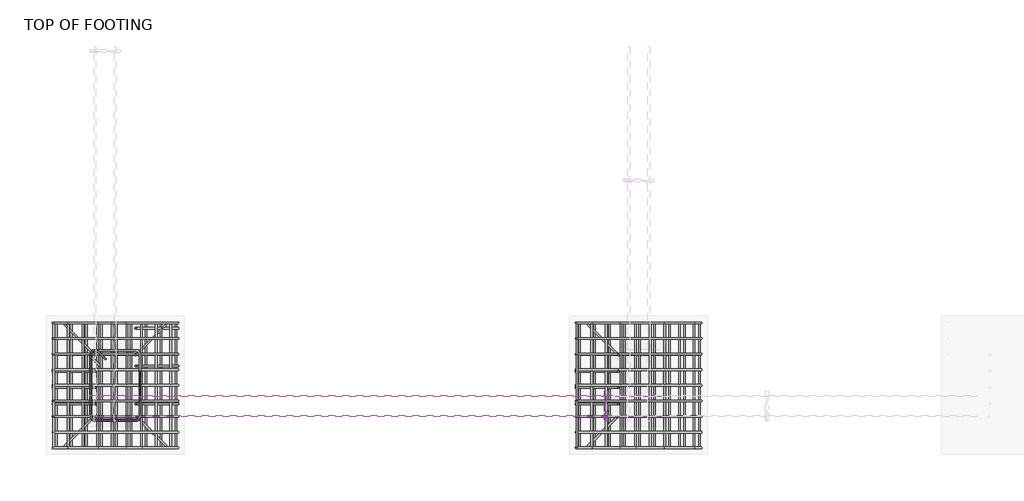
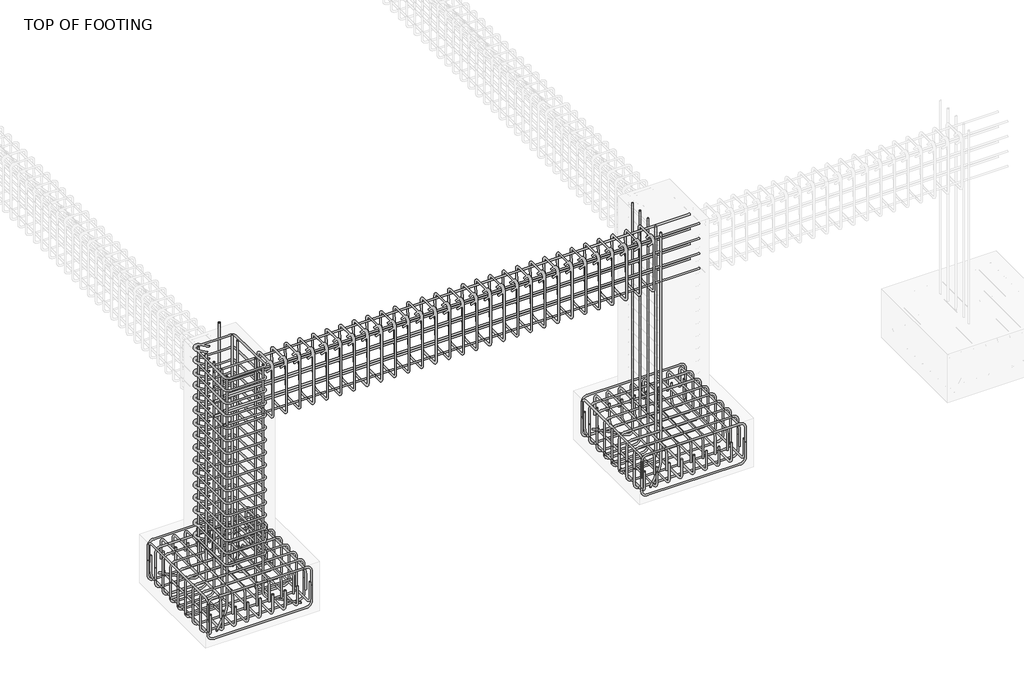
# One storey, part 2 of 9: 21 reinforcing bars.
"""IFC4 building model written with IfcOpenShell, lengths in millimetres."""

from ifc_helpers import new_model, si_unit, point, frame, origin, place, context, project, spatial, polyline, circle_curve, trimmed, segment, composite_curve, source, transform, mapped, element, save
from ifc_brep_helpers import swept_disk

model = new_model("IFC4")

# Units and contexts
model_context = context("Model", 3, world=origin())
ifc_project = project(units=[si_unit("LENGTHUNIT", "METRE", prefix="MILLI")], contexts=[model_context])

# Site, building, storey
site = spatial("IfcSite", under=ifc_project)
building = spatial("IfcBuilding", under=site)
storey = spatial("IfcBuildingStorey", under=building, Name="TOP OF FOOTING", Elevation=-1828.8)

# Reinforcing bars
placement = place(None, origin())
reinforcing_bar_shape = source(origin(), model_context, "Body", "SolidModel", [
    swept_disk(composite_curve([segment(polyline([(-11129.6174526, -598.6824927, -2052.8356656), (-11129.6174526, -598.6824927, -2200.1356656)]), True, "CONTINUOUS"), segment(trimmed(circle_curve(frame((-11175.9674526, -598.6824927, -2200.1356656), z_axis=(0.0, 1.0, 0.0), x_axis=(46.350000000000364, 0.0, 0.0)), 46.35), [point((-11129.6174526, -598.6824927, -2200.1356656))], [point((-11175.9674526, -598.6824927, -2246.4856656))], True, "CARTESIAN"), True, "CONTINUOUS"), segment(polyline([(-11175.9674526, -598.6824927, -2246.4856656), (-11990.5674526, -598.6824927, -2246.4856656)]), True, "CONTINUOUS"), segment(trimmed(circle_curve(frame((-11990.5674526, -598.6824927, -2200.1356656), z_axis=(0.0, 1.0, 0.0), x_axis=(0.0, 0.0, -46.350000000000364)), 46.35), [point((-11990.5674526, -598.6824927, -2246.4856656))], [point((-12036.9174526, -598.6824927, -2200.1356656))], True, "CARTESIAN"), True, "CONTINUOUS"), segment(polyline([(-12036.9174526, -598.6824927, -2200.1356656), (-12036.9174526, -598.6824927, -2052.8356656)]), True, "CONTINUOUS")], self_intersect=False), 6.35),
])
element("IfcReinforcingBar", 1, at=placement, inside=storey, context=model_context, shape_type="MappedRepresentation", body=[
    mapped(reinforcing_bar_shape, transform((0.0, 0.0, 0.0), x_axis=(1.0, 0.0, 0.0), y_axis=(0.0, 1.0, 0.0), z_axis=(0.0, 0.0, 1.0))),
    mapped(reinforcing_bar_shape, transform((0.0, -113.4125, 0.0), x_axis=(1.0, 0.0, 0.0), y_axis=(0.0, 1.0, 0.0), z_axis=(0.0, 0.0, 1.0))),
    mapped(reinforcing_bar_shape, transform((0.0, -226.825, 0.0), x_axis=(1.0, 0.0, 0.0), y_axis=(0.0, 1.0, 0.0), z_axis=(0.0, 0.0, 1.0))),
    mapped(reinforcing_bar_shape, transform((0.0, -340.2375, 0.0), x_axis=(1.0, 0.0, 0.0), y_axis=(0.0, 1.0, 0.0), z_axis=(0.0, 0.0, 1.0))),
    mapped(reinforcing_bar_shape, transform((0.0, -453.65, 0.0), x_axis=(1.0, 0.0, 0.0), y_axis=(0.0, 1.0, 0.0), z_axis=(0.0, 0.0, 1.0))),
    mapped(reinforcing_bar_shape, transform((0.0, -567.0625, 0.0), x_axis=(1.0, 0.0, 0.0), y_axis=(0.0, 1.0, 0.0), z_axis=(0.0, 0.0, 1.0))),
    mapped(reinforcing_bar_shape, transform((0.0, -680.475, 0.0), x_axis=(1.0, 0.0, 0.0), y_axis=(0.0, 1.0, 0.0), z_axis=(0.0, 0.0, 1.0))),
    mapped(reinforcing_bar_shape, transform((0.0, -793.8875, 0.0), x_axis=(1.0, 0.0, 0.0), y_axis=(0.0, 1.0, 0.0), z_axis=(0.0, 0.0, 1.0))),
    mapped(reinforcing_bar_shape, transform((0.0, -907.3, 0.0), x_axis=(1.0, 0.0, 0.0), y_axis=(0.0, 1.0, 0.0), z_axis=(0.0, 0.0, 1.0))),
])
reinforcing_bar_2_shape = source(origin(), model_context, "Body", "SolidModel", [
    swept_disk(composite_curve([segment(polyline([(-12036.9174526, -598.6824927, -2068.8), (-12036.9174526, -598.6824927, -1921.5)]), True, "CONTINUOUS"), segment(trimmed(circle_curve(frame((-11990.5674526, -598.6824927, -1921.5), z_axis=(0.0, 1.0, 0.0), x_axis=(-46.350000000000364, 0.0, 0.0)), 46.35), [point((-12036.9174526, -598.6824927, -1921.5))], [point((-11990.5674526, -598.6824927, -1875.15))], True, "CARTESIAN"), True, "CONTINUOUS"), segment(polyline([(-11990.5674526, -598.6824927, -1875.15), (-11175.9674526, -598.6824927, -1875.15)]), True, "CONTINUOUS"), segment(trimmed(circle_curve(frame((-11175.9674526, -598.6824927, -1921.5), z_axis=(0.0, 1.0, 0.0), x_axis=(0.0, 0.0, 46.34999999999991)), 46.35), [point((-11175.9674526, -598.6824927, -1875.15))], [point((-11129.6174526, -598.6824927, -1921.5))], True, "CARTESIAN"), True, "CONTINUOUS"), segment(polyline([(-11129.6174526, -598.6824927, -1921.5), (-11129.6174526, -598.6824927, -2068.8)]), True, "CONTINUOUS")], self_intersect=False), 6.35),
])
element("IfcReinforcingBar", 2, at=placement, inside=storey, context=model_context, shape_type="MappedRepresentation", body=[
    mapped(reinforcing_bar_2_shape, transform((0.0, 0.0, 0.0), x_axis=(1.0, 0.0, 0.0), y_axis=(0.0, 1.0, 0.0), z_axis=(0.0, 0.0, 1.0))),
    mapped(reinforcing_bar_2_shape, transform((0.0, -113.4125, 0.0), x_axis=(1.0, 0.0, 0.0), y_axis=(0.0, 1.0, 0.0), z_axis=(0.0, 0.0, 1.0))),
    mapped(reinforcing_bar_2_shape, transform((0.0, -226.825, 0.0), x_axis=(1.0, 0.0, 0.0), y_axis=(0.0, 1.0, 0.0), z_axis=(0.0, 0.0, 1.0))),
    mapped(reinforcing_bar_2_shape, transform((0.0, -340.2375, 0.0), x_axis=(1.0, 0.0, 0.0), y_axis=(0.0, 1.0, 0.0), z_axis=(0.0, 0.0, 1.0))),
    mapped(reinforcing_bar_2_shape, transform((0.0, -453.65, 0.0), x_axis=(1.0, 0.0, 0.0), y_axis=(0.0, 1.0, 0.0), z_axis=(0.0, 0.0, 1.0))),
    mapped(reinforcing_bar_2_shape, transform((0.0, -567.0625, 0.0), x_axis=(1.0, 0.0, 0.0), y_axis=(0.0, 1.0, 0.0), z_axis=(0.0, 0.0, 1.0))),
    mapped(reinforcing_bar_2_shape, transform((0.0, -680.475, 0.0), x_axis=(1.0, 0.0, 0.0), y_axis=(0.0, 1.0, 0.0), z_axis=(0.0, 0.0, 1.0))),
    mapped(reinforcing_bar_2_shape, transform((0.0, -793.8875, 0.0), x_axis=(1.0, 0.0, 0.0), y_axis=(0.0, 1.0, 0.0), z_axis=(0.0, 0.0, 1.0))),
    mapped(reinforcing_bar_2_shape, transform((0.0, -907.3, 0.0), x_axis=(1.0, 0.0, 0.0), y_axis=(0.0, 1.0, 0.0), z_axis=(0.0, 0.0, 1.0))),
])
reinforcing_bar_3_shape = source(origin(), model_context, "Body", "SolidModel", [
    swept_disk(composite_curve([segment(polyline([(-12013.2674526, -598.6824927, -2020.15), (-12013.2674526, -598.6824927, -2167.45)]), True, "CONTINUOUS"), segment(trimmed(circle_curve(frame((-12013.2674526, -645.0324927, -2167.45), z_axis=(-1.0, 0.0, 0.0), x_axis=(0.0, 46.35000000000002, 0.0)), 46.35), [point((-12013.2674526, -598.6824927, -2167.45))], [point((-12013.2674526, -645.0324927, -2213.8))], True, "CARTESIAN"), True, "CONTINUOUS"), segment(polyline([(-12013.2674526, -645.0324927, -2213.8), (-12013.2674526, -1459.6324927, -2213.8)]), True, "CONTINUOUS"), segment(trimmed(circle_curve(frame((-12013.2674526, -1459.6324927, -2167.45), z_axis=(-1.0, 0.0, 0.0), x_axis=(0.0, 0.0, -46.350000000000364)), 46.35), [point((-12013.2674526, -1459.6324927, -2213.8))], [point((-12013.2674526, -1505.9824927, -2167.45))], True, "CARTESIAN"), True, "CONTINUOUS"), segment(polyline([(-12013.2674526, -1505.9824927, -2167.45), (-12013.2674526, -1505.9824927, -2020.15)]), True, "CONTINUOUS")], self_intersect=False), 6.35),
])
element("IfcReinforcingBar", 3, at=placement, inside=storey, context=model_context, shape_type="MappedRepresentation", body=[
    mapped(reinforcing_bar_3_shape, transform((0.0, 0.0, 0.0), x_axis=(1.0, 0.0, 0.0), y_axis=(0.0, 1.0, 0.0), z_axis=(0.0, 0.0, 1.0))),
    mapped(reinforcing_bar_3_shape, transform((108.8370374, 0.0, 0.0), x_axis=(1.0, 0.0, 0.0), y_axis=(0.0, 1.0, 0.0), z_axis=(0.0, 0.0, 1.0))),
    mapped(reinforcing_bar_3_shape, transform((217.6740748, 0.0, 0.0), x_axis=(1.0, 0.0, 0.0), y_axis=(0.0, 1.0, 0.0), z_axis=(0.0, 0.0, 1.0))),
    mapped(reinforcing_bar_3_shape, transform((326.5111123, 0.0, 0.0), x_axis=(1.0, 0.0, 0.0), y_axis=(0.0, 1.0, 0.0), z_axis=(0.0, 0.0, 1.0))),
    mapped(reinforcing_bar_3_shape, transform((435.3481497, 0.0, 0.0), x_axis=(1.0, 0.0, 0.0), y_axis=(0.0, 1.0, 0.0), z_axis=(0.0, 0.0, 1.0))),
    mapped(reinforcing_bar_3_shape, transform((544.1851871, 0.0, 0.0), x_axis=(1.0, 0.0, 0.0), y_axis=(0.0, 1.0, 0.0), z_axis=(0.0, 0.0, 1.0))),
    mapped(reinforcing_bar_3_shape, transform((653.0222245, 0.0, 0.0), x_axis=(1.0, 0.0, 0.0), y_axis=(0.0, 1.0, 0.0), z_axis=(0.0, 0.0, 1.0))),
    mapped(reinforcing_bar_3_shape, transform((761.8592619, 0.0, 0.0), x_axis=(1.0, 0.0, 0.0), y_axis=(0.0, 1.0, 0.0), z_axis=(0.0, 0.0, 1.0))),
    mapped(reinforcing_bar_3_shape, transform((870.6962994, 0.0, 0.0), x_axis=(1.0, 0.0, 0.0), y_axis=(0.0, 1.0, 0.0), z_axis=(0.0, 0.0, 1.0))),
])
reinforcing_bar_4_shape = source(origin(), model_context, "Body", "SolidModel", [
    swept_disk(composite_curve([segment(polyline([(-11180.7455787, -598.6824927, -2076.9782245), (-11180.7455787, -598.6824927, -1929.6782245)]), True, "CONTINUOUS"), segment(trimmed(circle_curve(frame((-11180.7455787, -645.0324927, -1929.6782245), z_axis=(1.0, 0.0, 0.0), x_axis=(0.0, 46.35000000000002, 0.0)), 46.35), [point((-11180.7455787, -598.6824927, -1929.6782245))], [point((-11180.7455787, -645.0324927, -1883.3282245))], True, "CARTESIAN"), True, "CONTINUOUS"), segment(polyline([(-11180.7455787, -645.0324927, -1883.3282245), (-11180.7455787, -1459.6324927, -1883.3282245)]), True, "CONTINUOUS"), segment(trimmed(circle_curve(frame((-11180.7455787, -1459.6324927, -1929.6782245), z_axis=(1.0, 0.0, 0.0), x_axis=(0.0, 0.0, 46.34999999999991)), 46.35), [point((-11180.7455787, -1459.6324927, -1883.3282245))], [point((-11180.7455787, -1505.9824927, -1929.6782245))], True, "CARTESIAN"), True, "CONTINUOUS"), segment(polyline([(-11180.7455787, -1505.9824927, -1929.6782245), (-11180.7455787, -1505.9824927, -2076.9782245)]), True, "CONTINUOUS")], self_intersect=False), 6.35),
])
element("IfcReinforcingBar", 4, at=placement, inside=storey, context=model_context, shape_type="MappedRepresentation", body=[
    mapped(reinforcing_bar_4_shape, transform((0.0, 0.0, 0.0), x_axis=(1.0, 0.0, 0.0), y_axis=(0.0, 1.0, 0.0), z_axis=(0.0, 0.0, 1.0))),
    mapped(reinforcing_bar_4_shape, transform((-106.3275638, 0.0, 0.0), x_axis=(1.0, 0.0, 0.0), y_axis=(0.0, 1.0, 0.0), z_axis=(0.0, 0.0, 1.0))),
    mapped(reinforcing_bar_4_shape, transform((-212.6551275, 0.0, 0.0), x_axis=(1.0, 0.0, 0.0), y_axis=(0.0, 1.0, 0.0), z_axis=(0.0, 0.0, 1.0))),
    mapped(reinforcing_bar_4_shape, transform((-318.9826913, 0.0, 0.0), x_axis=(1.0, 0.0, 0.0), y_axis=(0.0, 1.0, 0.0), z_axis=(0.0, 0.0, 1.0))),
    mapped(reinforcing_bar_4_shape, transform((-425.310255, 0.0, 0.0), x_axis=(1.0, 0.0, 0.0), y_axis=(0.0, 1.0, 0.0), z_axis=(0.0, 0.0, 1.0))),
    mapped(reinforcing_bar_4_shape, transform((-531.6378188, 0.0, 0.0), x_axis=(1.0, 0.0, 0.0), y_axis=(0.0, 1.0, 0.0), z_axis=(0.0, 0.0, 1.0))),
    mapped(reinforcing_bar_4_shape, transform((-637.9653825, 0.0, 0.0), x_axis=(1.0, 0.0, 0.0), y_axis=(0.0, 1.0, 0.0), z_axis=(0.0, 0.0, 1.0))),
    mapped(reinforcing_bar_4_shape, transform((-744.2929463, 0.0, 0.0), x_axis=(1.0, 0.0, 0.0), y_axis=(0.0, 1.0, 0.0), z_axis=(0.0, 0.0, 1.0))),
    mapped(reinforcing_bar_4_shape, transform((-850.62051, 0.0, 0.0), x_axis=(1.0, 0.0, 0.0), y_axis=(0.0, 1.0, 0.0), z_axis=(0.0, 0.0, 1.0))),
])
reinforcing_bar_5_shape = source(origin(), model_context, "Body", "SolidModel", [
    swept_disk(composite_curve([segment(polyline([(-7329.6174526, -598.6824927, -2052.8356656), (-7329.6174526, -598.6824927, -2200.1356656)]), True, "CONTINUOUS"), segment(trimmed(circle_curve(frame((-7375.9674526, -598.6824927, -2200.1356656), z_axis=(0.0, 1.0, 0.0), x_axis=(46.349999999999454, 0.0, 0.0)), 46.35), [point((-7329.6174526, -598.6824927, -2200.1356656))], [point((-7375.9674526, -598.6824927, -2246.4856656))], True, "CARTESIAN"), True, "CONTINUOUS"), segment(polyline([(-7375.9674526, -598.6824927, -2246.4856656), (-8190.5674526, -598.6824927, -2246.4856656)]), True, "CONTINUOUS"), segment(trimmed(circle_curve(frame((-8190.5674526, -598.6824927, -2200.1356656), z_axis=(0.0, 1.0, 0.0), x_axis=(0.0, 0.0, -46.350000000000364)), 46.35), [point((-8190.5674526, -598.6824927, -2246.4856656))], [point((-8236.9174526, -598.6824927, -2200.1356656))], True, "CARTESIAN"), True, "CONTINUOUS"), segment(polyline([(-8236.9174526, -598.6824927, -2200.1356656), (-8236.9174526, -598.6824927, -2052.8356656)]), True, "CONTINUOUS")], self_intersect=False), 6.35),
])
element("IfcReinforcingBar", 5, at=placement, inside=storey, context=model_context, shape_type="MappedRepresentation", body=[
    mapped(reinforcing_bar_5_shape, transform((0.0, 0.0, 0.0), x_axis=(1.0, 0.0, 0.0), y_axis=(0.0, 1.0, 0.0), z_axis=(0.0, 0.0, 1.0))),
    mapped(reinforcing_bar_5_shape, transform((0.0, -113.4125, 0.0), x_axis=(1.0, 0.0, 0.0), y_axis=(0.0, 1.0, 0.0), z_axis=(0.0, 0.0, 1.0))),
    mapped(reinforcing_bar_5_shape, transform((0.0, -226.825, 0.0), x_axis=(1.0, 0.0, 0.0), y_axis=(0.0, 1.0, 0.0), z_axis=(0.0, 0.0, 1.0))),
    mapped(reinforcing_bar_5_shape, transform((0.0, -340.2375, 0.0), x_axis=(1.0, 0.0, 0.0), y_axis=(0.0, 1.0, 0.0), z_axis=(0.0, 0.0, 1.0))),
    mapped(reinforcing_bar_5_shape, transform((0.0, -453.65, 0.0), x_axis=(1.0, 0.0, 0.0), y_axis=(0.0, 1.0, 0.0), z_axis=(0.0, 0.0, 1.0))),
    mapped(reinforcing_bar_5_shape, transform((0.0, -567.0625, 0.0), x_axis=(1.0, 0.0, 0.0), y_axis=(0.0, 1.0, 0.0), z_axis=(0.0, 0.0, 1.0))),
    mapped(reinforcing_bar_5_shape, transform((0.0, -680.475, 0.0), x_axis=(1.0, 0.0, 0.0), y_axis=(0.0, 1.0, 0.0), z_axis=(0.0, 0.0, 1.0))),
    mapped(reinforcing_bar_5_shape, transform((0.0, -793.8875, 0.0), x_axis=(1.0, 0.0, 0.0), y_axis=(0.0, 1.0, 0.0), z_axis=(0.0, 0.0, 1.0))),
    mapped(reinforcing_bar_5_shape, transform((0.0, -907.3, 0.0), x_axis=(1.0, 0.0, 0.0), y_axis=(0.0, 1.0, 0.0), z_axis=(0.0, 0.0, 1.0))),
])
reinforcing_bar_6_shape = source(origin(), model_context, "Body", "SolidModel", [
    swept_disk(composite_curve([segment(polyline([(-8236.9174526, -598.6824927, -2068.8), (-8236.9174526, -598.6824927, -1921.5)]), True, "CONTINUOUS"), segment(trimmed(circle_curve(frame((-8190.5674526, -598.6824927, -1921.5), z_axis=(0.0, 1.0, 0.0), x_axis=(-46.350000000000364, 0.0, 0.0)), 46.35), [point((-8236.9174526, -598.6824927, -1921.5))], [point((-8190.5674526, -598.6824927, -1875.15))], True, "CARTESIAN"), True, "CONTINUOUS"), segment(polyline([(-8190.5674526, -598.6824927, -1875.15), (-7375.9674526, -598.6824927, -1875.15)]), True, "CONTINUOUS"), segment(trimmed(circle_curve(frame((-7375.9674526, -598.6824927, -1921.5), z_axis=(0.0, 1.0, 0.0), x_axis=(0.0, 0.0, 46.34999999999991)), 46.35), [point((-7375.9674526, -598.6824927, -1875.15))], [point((-7329.6174526, -598.6824927, -1921.5))], True, "CARTESIAN"), True, "CONTINUOUS"), segment(polyline([(-7329.6174526, -598.6824927, -1921.5), (-7329.6174526, -598.6824927, -2068.8)]), True, "CONTINUOUS")], self_intersect=False), 6.35),
])
element("IfcReinforcingBar", 6, at=placement, inside=storey, context=model_context, shape_type="MappedRepresentation", body=[
    mapped(reinforcing_bar_6_shape, transform((0.0, 0.0, 0.0), x_axis=(1.0, 0.0, 0.0), y_axis=(0.0, 1.0, 0.0), z_axis=(0.0, 0.0, 1.0))),
    mapped(reinforcing_bar_6_shape, transform((0.0, -113.4125, 0.0), x_axis=(1.0, 0.0, 0.0), y_axis=(0.0, 1.0, 0.0), z_axis=(0.0, 0.0, 1.0))),
    mapped(reinforcing_bar_6_shape, transform((0.0, -226.825, 0.0), x_axis=(1.0, 0.0, 0.0), y_axis=(0.0, 1.0, 0.0), z_axis=(0.0, 0.0, 1.0))),
    mapped(reinforcing_bar_6_shape, transform((0.0, -340.2375, 0.0), x_axis=(1.0, 0.0, 0.0), y_axis=(0.0, 1.0, 0.0), z_axis=(0.0, 0.0, 1.0))),
    mapped(reinforcing_bar_6_shape, transform((0.0, -453.65, 0.0), x_axis=(1.0, 0.0, 0.0), y_axis=(0.0, 1.0, 0.0), z_axis=(0.0, 0.0, 1.0))),
    mapped(reinforcing_bar_6_shape, transform((0.0, -567.0625, 0.0), x_axis=(1.0, 0.0, 0.0), y_axis=(0.0, 1.0, 0.0), z_axis=(0.0, 0.0, 1.0))),
    mapped(reinforcing_bar_6_shape, transform((0.0, -680.475, 0.0), x_axis=(1.0, 0.0, 0.0), y_axis=(0.0, 1.0, 0.0), z_axis=(0.0, 0.0, 1.0))),
    mapped(reinforcing_bar_6_shape, transform((0.0, -793.8875, 0.0), x_axis=(1.0, 0.0, 0.0), y_axis=(0.0, 1.0, 0.0), z_axis=(0.0, 0.0, 1.0))),
    mapped(reinforcing_bar_6_shape, transform((0.0, -907.3, 0.0), x_axis=(1.0, 0.0, 0.0), y_axis=(0.0, 1.0, 0.0), z_axis=(0.0, 0.0, 1.0))),
])
reinforcing_bar_7_shape = source(origin(), model_context, "Body", "SolidModel", [
    swept_disk(composite_curve([segment(polyline([(-8213.2674526, -598.6824927, -2020.15), (-8213.2674526, -598.6824927, -2167.45)]), True, "CONTINUOUS"), segment(trimmed(circle_curve(frame((-8213.2674526, -645.0324927, -2167.45), z_axis=(-1.0, 0.0, 0.0), x_axis=(0.0, 46.35000000000002, 0.0)), 46.35), [point((-8213.2674526, -598.6824927, -2167.45))], [point((-8213.2674526, -645.0324927, -2213.8))], True, "CARTESIAN"), True, "CONTINUOUS"), segment(polyline([(-8213.2674526, -645.0324927, -2213.8), (-8213.2674526, -1459.6324927, -2213.8)]), True, "CONTINUOUS"), segment(trimmed(circle_curve(frame((-8213.2674526, -1459.6324927, -2167.45), z_axis=(-1.0, 0.0, 0.0), x_axis=(0.0, 0.0, -46.350000000000364)), 46.35), [point((-8213.2674526, -1459.6324927, -2213.8))], [point((-8213.2674526, -1505.9824927, -2167.45))], True, "CARTESIAN"), True, "CONTINUOUS"), segment(polyline([(-8213.2674526, -1505.9824927, -2167.45), (-8213.2674526, -1505.9824927, -2020.15)]), True, "CONTINUOUS")], self_intersect=False), 6.35),
])
element("IfcReinforcingBar", 7, at=placement, inside=storey, context=model_context, shape_type="MappedRepresentation", body=[
    mapped(reinforcing_bar_7_shape, transform((0.0, 0.0, 0.0), x_axis=(1.0, 0.0, 0.0), y_axis=(0.0, 1.0, 0.0), z_axis=(0.0, 0.0, 1.0))),
    mapped(reinforcing_bar_7_shape, transform((108.8370374, 0.0, 0.0), x_axis=(1.0, 0.0, 0.0), y_axis=(0.0, 1.0, 0.0), z_axis=(0.0, 0.0, 1.0))),
    mapped(reinforcing_bar_7_shape, transform((217.6740748, 0.0, 0.0), x_axis=(1.0, 0.0, 0.0), y_axis=(0.0, 1.0, 0.0), z_axis=(0.0, 0.0, 1.0))),
    mapped(reinforcing_bar_7_shape, transform((326.5111123, 0.0, 0.0), x_axis=(1.0, 0.0, 0.0), y_axis=(0.0, 1.0, 0.0), z_axis=(0.0, 0.0, 1.0))),
    mapped(reinforcing_bar_7_shape, transform((435.3481497, 0.0, 0.0), x_axis=(1.0, 0.0, 0.0), y_axis=(0.0, 1.0, 0.0), z_axis=(0.0, 0.0, 1.0))),
    mapped(reinforcing_bar_7_shape, transform((544.1851871, 0.0, 0.0), x_axis=(1.0, 0.0, 0.0), y_axis=(0.0, 1.0, 0.0), z_axis=(0.0, 0.0, 1.0))),
    mapped(reinforcing_bar_7_shape, transform((653.0222245, 0.0, 0.0), x_axis=(1.0, 0.0, 0.0), y_axis=(0.0, 1.0, 0.0), z_axis=(0.0, 0.0, 1.0))),
    mapped(reinforcing_bar_7_shape, transform((761.8592619, 0.0, 0.0), x_axis=(1.0, 0.0, 0.0), y_axis=(0.0, 1.0, 0.0), z_axis=(0.0, 0.0, 1.0))),
    mapped(reinforcing_bar_7_shape, transform((870.6962994, 0.0, 0.0), x_axis=(1.0, 0.0, 0.0), y_axis=(0.0, 1.0, 0.0), z_axis=(0.0, 0.0, 1.0))),
])
reinforcing_bar_8_shape = source(origin(), model_context, "Body", "SolidModel", [
    swept_disk(composite_curve([segment(polyline([(-7380.7455787, -598.6824927, -2076.9782245), (-7380.7455787, -598.6824927, -1929.6782245)]), True, "CONTINUOUS"), segment(trimmed(circle_curve(frame((-7380.7455787, -645.0324927, -1929.6782245), z_axis=(1.0, 0.0, 0.0), x_axis=(0.0, 46.35000000000002, 0.0)), 46.35), [point((-7380.7455787, -598.6824927, -1929.6782245))], [point((-7380.7455787, -645.0324927, -1883.3282245))], True, "CARTESIAN"), True, "CONTINUOUS"), segment(polyline([(-7380.7455787, -645.0324927, -1883.3282245), (-7380.7455787, -1459.6324927, -1883.3282245)]), True, "CONTINUOUS"), segment(trimmed(circle_curve(frame((-7380.7455787, -1459.6324927, -1929.6782245), z_axis=(1.0, 0.0, 0.0), x_axis=(0.0, 0.0, 46.34999999999991)), 46.35), [point((-7380.7455787, -1459.6324927, -1883.3282245))], [point((-7380.7455787, -1505.9824927, -1929.6782245))], True, "CARTESIAN"), True, "CONTINUOUS"), segment(polyline([(-7380.7455787, -1505.9824927, -1929.6782245), (-7380.7455787, -1505.9824927, -2076.9782245)]), True, "CONTINUOUS")], self_intersect=False), 6.35),
])
element("IfcReinforcingBar", 8, at=placement, inside=storey, context=model_context, shape_type="MappedRepresentation", body=[
    mapped(reinforcing_bar_8_shape, transform((0.0, 0.0, 0.0), x_axis=(1.0, 0.0, 0.0), y_axis=(0.0, 1.0, 0.0), z_axis=(0.0, 0.0, 1.0))),
    mapped(reinforcing_bar_8_shape, transform((-106.3275638, 0.0, 0.0), x_axis=(1.0, 0.0, 0.0), y_axis=(0.0, 1.0, 0.0), z_axis=(0.0, 0.0, 1.0))),
    mapped(reinforcing_bar_8_shape, transform((-212.6551275, 0.0, 0.0), x_axis=(1.0, 0.0, 0.0), y_axis=(0.0, 1.0, 0.0), z_axis=(0.0, 0.0, 1.0))),
    mapped(reinforcing_bar_8_shape, transform((-318.9826913, 0.0, 0.0), x_axis=(1.0, 0.0, 0.0), y_axis=(0.0, 1.0, 0.0), z_axis=(0.0, 0.0, 1.0))),
    mapped(reinforcing_bar_8_shape, transform((-425.310255, 0.0, 0.0), x_axis=(1.0, 0.0, 0.0), y_axis=(0.0, 1.0, 0.0), z_axis=(0.0, 0.0, 1.0))),
    mapped(reinforcing_bar_8_shape, transform((-531.6378188, 0.0, 0.0), x_axis=(1.0, 0.0, 0.0), y_axis=(0.0, 1.0, 0.0), z_axis=(0.0, 0.0, 1.0))),
    mapped(reinforcing_bar_8_shape, transform((-637.9653825, 0.0, 0.0), x_axis=(1.0, 0.0, 0.0), y_axis=(0.0, 1.0, 0.0), z_axis=(0.0, 0.0, 1.0))),
    mapped(reinforcing_bar_8_shape, transform((-744.2929463, 0.0, 0.0), x_axis=(1.0, 0.0, 0.0), y_axis=(0.0, 1.0, 0.0), z_axis=(0.0, 0.0, 1.0))),
    mapped(reinforcing_bar_8_shape, transform((-850.62051, 0.0, 0.0), x_axis=(1.0, 0.0, 0.0), y_axis=(0.0, 1.0, 0.0), z_axis=(0.0, 0.0, 1.0))),
])
reinforcing_bar_9_shape = source(origin(), model_context, "Body", "SolidModel", [
    swept_disk(composite_curve([segment(polyline([(-11730.5674526, -1187.8357134, -40.0), (-11730.5674526, -1187.8357134, -2148.1729582)]), True, "CONTINUOUS"), segment(trimmed(circle_curve(frame((-11776.9174526, -1187.8357134, -2148.1729582), z_axis=(0.0, 1.0, 0.0), x_axis=(46.350000000000364, 0.0, 0.0)), 46.35), [point((-11730.5674526, -1187.8357134, -2148.1729582))], [point((-11776.9174526, -1187.8357134, -2194.5229582))], True, "CARTESIAN"), True, "CONTINUOUS"), segment(polyline([(-11776.9174526, -1187.8357134, -2194.5229582), (-12043.513478, -1187.8357134, -2194.5229582)]), True, "CONTINUOUS")], self_intersect=False), 6.35),
])
element("IfcReinforcingBar", 9, at=placement, inside=storey, context=model_context, shape_type="MappedRepresentation", body=[
    mapped(reinforcing_bar_9_shape, transform((0.0, 0.0, 0.0), x_axis=(1.0, 0.0, 0.0), y_axis=(0.0, 1.0, 0.0), z_axis=(0.0, 0.0, 1.0))),
    mapped(reinforcing_bar_9_shape, transform((0.0, 119.1364467, 0.0), x_axis=(1.0, 0.0, 0.0), y_axis=(0.0, 1.0, 0.0), z_axis=(0.0, 0.0, 1.0))),
    mapped(reinforcing_bar_9_shape, transform((0.0, 238.2728934, 0.0), x_axis=(1.0, 0.0, 0.0), y_axis=(0.0, 1.0, 0.0), z_axis=(0.0, 0.0, 1.0))),
])
reinforcing_bar_10_shape = source(origin(), model_context, "Body", "SolidModel", [
    swept_disk(composite_curve([segment(polyline([(-11652.6560921, -863.6082581, -1782.45), (-11708.399655, -807.8646951, -1782.45)]), True, "CONTINUOUS"), segment(trimmed(circle_curve(frame((-11730.5674526, -830.0324927, -1782.45), z_axis=(0.0, 0.0, 1.0), x_axis=(22.167797600000995, 22.167797600000085, 0.0)), 31.35), [point((-11708.399655, -807.8646951, -1782.45))], [point((-11761.9174526, -830.0324927, -1782.45))], True, "CARTESIAN"), True, "CONTINUOUS"), segment(polyline([(-11761.9174526, -830.0324927, -1782.45), (-11761.9174526, -1274.6324927, -1782.45)]), True, "CONTINUOUS"), segment(trimmed(circle_curve(frame((-11730.5674526, -1274.6324927, -1782.45), z_axis=(0.0, 0.0, 1.0), x_axis=(-31.350000000000364, 0.0, 0.0)), 31.35), [point((-11761.9174526, -1274.6324927, -1782.45))], [point((-11730.5674526, -1305.9824927, -1782.45))], True, "CARTESIAN"), True, "CONTINUOUS"), segment(polyline([(-11730.5674526, -1305.9824927, -1782.45), (-11435.9674526, -1305.9824927, -1782.45)]), True, "CONTINUOUS"), segment(trimmed(circle_curve(frame((-11435.9674526, -1274.642312, -1783.2345856), z_axis=(0.0, 0.025026655153786315, 0.9996867842138424), x_axis=(0.0, -31.34018070000002, 0.7845855999999003)), 31.35), [point((-11435.9674526, -1305.9824927, -1782.45))], [point((-11404.6174526, -1274.642312, -1783.2345856))], True, "CARTESIAN"), True, "CONTINUOUS"), segment(polyline([(-11404.6174526, -1274.642312, -1783.2345856), (-11404.6174526, -830.0226734, -1794.3654144)]), True, "CONTINUOUS"), segment(trimmed(circle_curve(frame((-11435.9674526, -830.0226734, -1794.3654144), z_axis=(0.0, 0.025026655153786315, 0.9996867842138424), x_axis=(31.350000000000364, 0.0, 0.0)), 31.35), [point((-11404.6174526, -830.0226734, -1794.3654144))], [point((-11435.9674526, -798.6824927, -1795.15))], True, "CARTESIAN"), True, "CONTINUOUS"), segment(polyline([(-11435.9674526, -798.6824927, -1795.15), (-11730.5674526, -798.6824927, -1795.15)]), True, "CONTINUOUS"), segment(trimmed(circle_curve(frame((-11730.5674526, -830.0324927, -1795.15), z_axis=(0.0, 0.0, 1.0), x_axis=(0.0, 31.350000000000023, 0.0)), 31.35), [point((-11730.5674526, -798.6824927, -1795.15))], [point((-11752.7352502, -852.2002903, -1795.15))], True, "CARTESIAN"), True, "CONTINUOUS"), segment(polyline([(-11752.7352502, -852.2002903, -1795.15), (-11696.9916873, -907.9438533, -1795.15)]), True, "CONTINUOUS")], self_intersect=False), 6.35),
])
element("IfcReinforcingBar", 10, at=placement, inside=storey, context=model_context, shape_type="MappedRepresentation", body=[
    mapped(reinforcing_bar_10_shape, transform((0.0, 0.0, 0.0), x_axis=(1.0, 0.0, 0.0), y_axis=(0.0, 1.0, 0.0), z_axis=(0.0, 0.0, 1.0))),
    mapped(reinforcing_bar_10_shape, transform((0.0, 0.0, 115.74), x_axis=(1.0, 0.0, 0.0), y_axis=(0.0, 1.0, 0.0), z_axis=(0.0, 0.0, 1.0))),
    mapped(reinforcing_bar_10_shape, transform((0.0, 0.0, 231.48), x_axis=(1.0, 0.0, 0.0), y_axis=(0.0, 1.0, 0.0), z_axis=(0.0, 0.0, 1.0))),
    mapped(reinforcing_bar_10_shape, transform((0.0, 0.0, 347.22), x_axis=(1.0, 0.0, 0.0), y_axis=(0.0, 1.0, 0.0), z_axis=(0.0, 0.0, 1.0))),
    mapped(reinforcing_bar_10_shape, transform((0.0, 0.0, 462.96), x_axis=(1.0, 0.0, 0.0), y_axis=(0.0, 1.0, 0.0), z_axis=(0.0, 0.0, 1.0))),
    mapped(reinforcing_bar_10_shape, transform((0.0, 0.0, 578.7), x_axis=(1.0, 0.0, 0.0), y_axis=(0.0, 1.0, 0.0), z_axis=(0.0, 0.0, 1.0))),
    mapped(reinforcing_bar_10_shape, transform((0.0, 0.0, 694.44), x_axis=(1.0, 0.0, 0.0), y_axis=(0.0, 1.0, 0.0), z_axis=(0.0, 0.0, 1.0))),
    mapped(reinforcing_bar_10_shape, transform((0.0, 0.0, 810.18), x_axis=(1.0, 0.0, 0.0), y_axis=(0.0, 1.0, 0.0), z_axis=(0.0, 0.0, 1.0))),
    mapped(reinforcing_bar_10_shape, transform((0.0, 0.0, 925.92), x_axis=(1.0, 0.0, 0.0), y_axis=(0.0, 1.0, 0.0), z_axis=(0.0, 0.0, 1.0))),
    mapped(reinforcing_bar_10_shape, transform((0.0, 0.0, 1041.66), x_axis=(1.0, 0.0, 0.0), y_axis=(0.0, 1.0, 0.0), z_axis=(0.0, 0.0, 1.0))),
    mapped(reinforcing_bar_10_shape, transform((0.0, 0.0, 1157.4), x_axis=(1.0, 0.0, 0.0), y_axis=(0.0, 1.0, 0.0), z_axis=(0.0, 0.0, 1.0))),
    mapped(reinforcing_bar_10_shape, transform((0.0, 0.0, 1273.14), x_axis=(1.0, 0.0, 0.0), y_axis=(0.0, 1.0, 0.0), z_axis=(0.0, 0.0, 1.0))),
    mapped(reinforcing_bar_10_shape, transform((0.0, 0.0, 1388.88), x_axis=(1.0, 0.0, 0.0), y_axis=(0.0, 1.0, 0.0), z_axis=(0.0, 0.0, 1.0))),
    mapped(reinforcing_bar_10_shape, transform((0.0, 0.0, 1504.62), x_axis=(1.0, 0.0, 0.0), y_axis=(0.0, 1.0, 0.0), z_axis=(0.0, 0.0, 1.0))),
    mapped(reinforcing_bar_10_shape, transform((0.0, 0.0, 1620.36), x_axis=(1.0, 0.0, 0.0), y_axis=(0.0, 1.0, 0.0), z_axis=(0.0, 0.0, 1.0))),
    mapped(reinforcing_bar_10_shape, transform((0.0, 0.0, 1736.1), x_axis=(1.0, 0.0, 0.0), y_axis=(0.0, 1.0, 0.0), z_axis=(0.0, 0.0, 1.0))),
])
element("IfcReinforcingBar", 11, at=placement, inside=storey, context=model_context, shape_type="SolidModel", body=[
    swept_disk(composite_curve([segment(polyline([(-11730.5674526, -832.8986176, -40.0), (-11730.5674526, -832.8986176, -2148.1729582)]), True, "CONTINUOUS"), segment(trimmed(circle_curve(frame((-11763.3418519, -800.1242183, -2148.1729582), z_axis=(0.7071067811865507, 0.7071067811865444, 0.0), x_axis=(32.77439930000037, -32.774399299999914, 0.0)), 46.35), [point((-11730.5674526, -832.8986176, -2148.1729582))], [point((-11763.3418519, -800.1242183, -2194.5229582))], True, "CARTESIAN"), True, "CONTINUOUS"), segment(polyline([(-11763.3418519, -800.1242183, -2194.5229582), (-11951.8537093, -611.6123609, -2194.5229582)]), True, "CONTINUOUS")], self_intersect=False), 6.35),
])
element("IfcReinforcingBar", 12, at=placement, inside=storey, context=model_context, shape_type="SolidModel", body=[
    swept_disk(composite_curve([segment(polyline([(-11740.5132324, -1281.7121476, -40.0), (-11740.5132324, -1281.7121476, -2148.1729582)]), True, "CONTINUOUS"), segment(trimmed(circle_curve(frame((-11773.2876317, -1314.4865469, -2148.1729582), z_axis=(-0.707106781186547, 0.707106781186548, 0.0), x_axis=(32.77439929999855, 32.774399299999914, 0.0)), 46.35), [point((-11740.5132324, -1281.7121476, -2148.1729582))], [point((-11773.2876317, -1314.4865469, -2194.5229582))], True, "CARTESIAN"), True, "CONTINUOUS"), segment(polyline([(-11773.2876317, -1314.4865469, -2194.5229582), (-11951.8537093, -1493.0526245, -2194.5229582)]), True, "CONTINUOUS")], self_intersect=False), 6.35),
])
element("IfcReinforcingBar", 13, at=placement, inside=storey, context=model_context, shape_type="SolidModel", body=[
    swept_disk(composite_curve([segment(polyline([(-11435.9674526, -832.8986176, -40.0), (-11435.9674526, -832.8986176, -2148.1729582)]), True, "CONTINUOUS"), segment(trimmed(circle_curve(frame((-11403.1930533, -800.1242183, -2148.1729582), z_axis=(0.7071067811865507, -0.7071067811865444, 0.0), x_axis=(-32.77439930000037, -32.774399299999914, 0.0)), 46.35), [point((-11435.9674526, -832.8986176, -2148.1729582))], [point((-11403.1930533, -800.1242183, -2194.5229582))], True, "CARTESIAN"), True, "CONTINUOUS"), segment(polyline([(-11403.1930533, -800.1242183, -2194.5229582), (-11214.6811959, -611.6123609, -2194.5229582)]), True, "CONTINUOUS")], self_intersect=False), 6.35),
])
element("IfcReinforcingBar", 14, at=placement, inside=storey, context=model_context, shape_type="SolidModel", body=[
    swept_disk(composite_curve([segment(polyline([(-11426.0216728, -1281.7121476, -40.0), (-11426.0216728, -1281.7121476, -2148.1729582)]), True, "CONTINUOUS"), segment(trimmed(circle_curve(frame((-11393.2472735, -1314.4865469, -2148.1729582), z_axis=(-0.707106781186547, -0.707106781186548, 0.0), x_axis=(-32.77439930000037, 32.774399299999914, 0.0)), 46.35), [point((-11426.0216728, -1281.7121476, -2148.1729582))], [point((-11393.2472735, -1314.4865469, -2194.5229582))], True, "CARTESIAN"), True, "CONTINUOUS"), segment(polyline([(-11393.2472735, -1314.4865469, -2194.5229582), (-11214.6811959, -1493.0526245, -2194.5229582)]), True, "CONTINUOUS")], self_intersect=False), 6.35),
])
reinforcing_bar_11_shape = source(origin(), model_context, "Body", "SolidModel", [
    swept_disk(composite_curve([segment(polyline([(-11435.9674526, -1187.8357134, -40.0), (-11435.9674526, -1187.8357134, -2148.1729582)]), True, "CONTINUOUS"), segment(trimmed(circle_curve(frame((-11389.6174526, -1187.8357134, -2148.1729582), z_axis=(0.0, -1.0, 0.0), x_axis=(-46.350000000000364, 0.0, 0.0)), 46.35), [point((-11435.9674526, -1187.8357134, -2148.1729582))], [point((-11389.6174526, -1187.8357134, -2194.5229582))], True, "CARTESIAN"), True, "CONTINUOUS"), segment(polyline([(-11389.6174526, -1187.8357134, -2194.5229582), (-11123.0214272, -1187.8357134, -2194.5229582)]), True, "CONTINUOUS")], self_intersect=False), 6.35),
])
element("IfcReinforcingBar", 15, at=placement, inside=storey, context=model_context, shape_type="MappedRepresentation", body=[
    mapped(reinforcing_bar_11_shape, transform((0.0, 0.0, 0.0), x_axis=(1.0, 0.0, 0.0), y_axis=(0.0, 1.0, 0.0), z_axis=(0.0, 0.0, 1.0))),
    mapped(reinforcing_bar_11_shape, transform((0.0, 275.486447, 0.0), x_axis=(1.0, 0.0, 0.0), y_axis=(0.0, 1.0, 0.0), z_axis=(0.0, 0.0, 1.0))),
    mapped(reinforcing_bar_11_shape, transform((0.0, 550.972894, 0.0), x_axis=(1.0, 0.0, 0.0), y_axis=(0.0, 1.0, 0.0), z_axis=(0.0, 0.0, 1.0))),
])
reinforcing_bar_12_shape = source(origin(), model_context, "Body", "SolidModel", [
    swept_disk(composite_curve([segment(polyline([(-7930.5674526, -1187.8357134, -40.0), (-7930.5674526, -1187.8357134, -2148.1729582)]), True, "CONTINUOUS"), segment(trimmed(circle_curve(frame((-7976.9174526, -1187.8357134, -2148.1729582), z_axis=(0.0, 1.0, 0.0), x_axis=(46.349999999999454, 0.0, 0.0)), 46.35), [point((-7930.5674526, -1187.8357134, -2148.1729582))], [point((-7976.9174526, -1187.8357134, -2194.5229582))], True, "CARTESIAN"), True, "CONTINUOUS"), segment(polyline([(-7976.9174526, -1187.8357134, -2194.5229582), (-8243.513478, -1187.8357134, -2194.5229582)]), True, "CONTINUOUS")], self_intersect=False), 6.35),
])
element("IfcReinforcingBar", 16, at=placement, inside=storey, context=model_context, shape_type="MappedRepresentation", body=[
    mapped(reinforcing_bar_12_shape, transform((0.0, 0.0, 0.0), x_axis=(1.0, 0.0, 0.0), y_axis=(0.0, 1.0, 0.0), z_axis=(0.0, 0.0, 1.0))),
    mapped(reinforcing_bar_12_shape, transform((0.0, 119.1364467, 0.0), x_axis=(1.0, 0.0, 0.0), y_axis=(0.0, 1.0, 0.0), z_axis=(0.0, 0.0, 1.0))),
    mapped(reinforcing_bar_12_shape, transform((0.0, 238.2728934, 0.0), x_axis=(1.0, 0.0, 0.0), y_axis=(0.0, 1.0, 0.0), z_axis=(0.0, 0.0, 1.0))),
])
element("IfcReinforcingBar", 17, at=placement, inside=storey, context=model_context, shape_type="SolidModel", body=[
    swept_disk(composite_curve([segment(polyline([(-7930.5674526, -832.8986176, -40.0), (-7930.5674526, -832.8986176, -2148.1729582)]), True, "CONTINUOUS"), segment(trimmed(circle_curve(frame((-7963.3418519, -800.1242183, -2148.1729582), z_axis=(0.7071067811865507, 0.7071067811865444, 0.0), x_axis=(32.77439929999946, -32.774399299999914, 0.0)), 46.35), [point((-7930.5674526, -832.8986176, -2148.1729582))], [point((-7963.3418519, -800.1242183, -2194.5229582))], True, "CARTESIAN"), True, "CONTINUOUS"), segment(polyline([(-7963.3418519, -800.1242183, -2194.5229582), (-8151.8537093, -611.6123609, -2194.5229582)]), True, "CONTINUOUS")], self_intersect=False), 6.35),
])
element("IfcReinforcingBar", 18, at=placement, inside=storey, context=model_context, shape_type="SolidModel", body=[
    swept_disk(composite_curve([segment(polyline([(-7940.5132324, -1281.7121476, -40.0), (-7940.5132324, -1281.7121476, -2148.1729582)]), True, "CONTINUOUS"), segment(trimmed(circle_curve(frame((-7973.2876317, -1314.4865469, -2148.1729582), z_axis=(-0.707106781186547, 0.707106781186548, 0.0), x_axis=(32.77439930000037, 32.774399299999914, 0.0)), 46.35), [point((-7940.5132324, -1281.7121476, -2148.1729582))], [point((-7973.2876317, -1314.4865469, -2194.5229582))], True, "CARTESIAN"), True, "CONTINUOUS"), segment(polyline([(-7973.2876317, -1314.4865469, -2194.5229582), (-8151.8537093, -1493.0526245, -2194.5229582)]), True, "CONTINUOUS")], self_intersect=False), 6.35),
])
reinforcing_bar_13_shape = source(origin(), model_context, "Body", "SolidModel", [
    swept_disk(composite_curve([segment(polyline([(-11351.9174526, -1196.7211322, -111.2757654), (-11351.9174526, -1252.4646951, -55.5322024)]), True, "CONTINUOUS"), segment(trimmed(circle_curve(frame((-11351.9174526, -1274.6324927, -77.7), z_axis=(1.0, 0.0, 0.0), x_axis=(0.0, 22.167797600000085, 22.1677976)), 31.35), [point((-11351.9174526, -1252.4646951, -55.5322024))], [point((-11351.9174526, -1305.9824927, -77.7))], True, "CARTESIAN"), True, "CONTINUOUS"), segment(polyline([(-11351.9174526, -1305.9824927, -77.7), (-11351.9174526, -1305.9824927, -522.3)]), True, "CONTINUOUS"), segment(trimmed(circle_curve(frame((-11351.9174526, -1274.6324927, -522.3), z_axis=(1.0, 0.0, 0.0), x_axis=(0.0, -31.34999999999991, 0.0)), 31.35), [point((-11351.9174526, -1305.9824927, -522.3))], [point((-11351.9174526, -1274.6324927, -553.65))], True, "CARTESIAN"), True, "CONTINUOUS"), segment(polyline([(-11351.9174526, -1274.6324927, -553.65), (-11351.9174526, -1130.0324927, -553.65)]), True, "CONTINUOUS"), segment(trimmed(circle_curve(frame((-11352.7020383, -1130.0324927, -522.3098193), z_axis=(0.9996867842138424, 0.0, 0.025026655153786322), x_axis=(0.7845856999992975, 0.0, -31.34018070000002)), 31.35), [point((-11351.9174526, -1130.0324927, -553.65))], [point((-11352.7020383, -1098.6824927, -522.3098193))], True, "CARTESIAN"), True, "CONTINUOUS"), segment(polyline([(-11352.7020383, -1098.6824927, -522.3098193), (-11363.832867, -1098.6824927, -77.6901807)]), True, "CONTINUOUS"), segment(trimmed(circle_curve(frame((-11363.832867, -1130.0324927, -77.6901807), z_axis=(0.9996867842138424, 0.0, 0.025026655153786322), x_axis=(0.0, 31.34999999999991, 0.0)), 31.35), [point((-11363.832867, -1098.6824927, -77.6901807))], [point((-11364.6174526, -1130.0324927, -46.35))], True, "CARTESIAN"), True, "CONTINUOUS"), segment(polyline([(-11364.6174526, -1130.0324927, -46.35), (-11364.6174526, -1274.6324927, -46.35)]), True, "CONTINUOUS"), segment(trimmed(circle_curve(frame((-11364.6174526, -1274.6324927, -77.7), z_axis=(1.0, 0.0, 0.0), x_axis=(0.0, 0.0, 31.35)), 31.35), [point((-11364.6174526, -1274.6324927, -46.35))], [point((-11364.6174526, -1296.8002903, -99.8677976))], True, "CARTESIAN"), True, "CONTINUOUS"), segment(polyline([(-11364.6174526, -1296.8002903, -99.8677976), (-11364.6174526, -1241.0567274, -155.6113605)]), True, "CONTINUOUS")], self_intersect=False), 6.35),
])
element("IfcReinforcingBar", 19, at=placement, inside=storey, context=model_context, shape_type="MappedRepresentation", body=[
    mapped(reinforcing_bar_13_shape, transform((0.0, 0.0, 0.0), x_axis=(1.0, 0.0, 0.0), y_axis=(0.0, 1.0, 0.0), z_axis=(0.0, 0.0, 1.0))),
    mapped(reinforcing_bar_13_shape, transform((119.1892857, 0.0, 0.0), x_axis=(1.0, 0.0, 0.0), y_axis=(0.0, 1.0, 0.0), z_axis=(0.0, 0.0, 1.0))),
    mapped(reinforcing_bar_13_shape, transform((238.3785714, 0.0, 0.0), x_axis=(1.0, 0.0, 0.0), y_axis=(0.0, 1.0, 0.0), z_axis=(0.0, 0.0, 1.0))),
    mapped(reinforcing_bar_13_shape, transform((357.5678571, 0.0, 0.0), x_axis=(1.0, 0.0, 0.0), y_axis=(0.0, 1.0, 0.0), z_axis=(0.0, 0.0, 1.0))),
    mapped(reinforcing_bar_13_shape, transform((476.7571429, 0.0, 0.0), x_axis=(1.0, 0.0, 0.0), y_axis=(0.0, 1.0, 0.0), z_axis=(0.0, 0.0, 1.0))),
    mapped(reinforcing_bar_13_shape, transform((595.9464286, 0.0, 0.0), x_axis=(1.0, 0.0, 0.0), y_axis=(0.0, 1.0, 0.0), z_axis=(0.0, 0.0, 1.0))),
    mapped(reinforcing_bar_13_shape, transform((715.1357143, 0.0, 0.0), x_axis=(1.0, 0.0, 0.0), y_axis=(0.0, 1.0, 0.0), z_axis=(0.0, 0.0, 1.0))),
    mapped(reinforcing_bar_13_shape, transform((834.325, 0.0, 0.0), x_axis=(1.0, 0.0, 0.0), y_axis=(0.0, 1.0, 0.0), z_axis=(0.0, 0.0, 1.0))),
    mapped(reinforcing_bar_13_shape, transform((953.5142857, 0.0, 0.0), x_axis=(1.0, 0.0, 0.0), y_axis=(0.0, 1.0, 0.0), z_axis=(0.0, 0.0, 1.0))),
    mapped(reinforcing_bar_13_shape, transform((1072.7035714, 0.0, 0.0), x_axis=(1.0, 0.0, 0.0), y_axis=(0.0, 1.0, 0.0), z_axis=(0.0, 0.0, 1.0))),
    mapped(reinforcing_bar_13_shape, transform((1191.8928571, 0.0, 0.0), x_axis=(1.0, 0.0, 0.0), y_axis=(0.0, 1.0, 0.0), z_axis=(0.0, 0.0, 1.0))),
    mapped(reinforcing_bar_13_shape, transform((1311.0821429, 0.0, 0.0), x_axis=(1.0, 0.0, 0.0), y_axis=(0.0, 1.0, 0.0), z_axis=(0.0, 0.0, 1.0))),
    mapped(reinforcing_bar_13_shape, transform((1430.2714286, 0.0, 0.0), x_axis=(1.0, 0.0, 0.0), y_axis=(0.0, 1.0, 0.0), z_axis=(0.0, 0.0, 1.0))),
    mapped(reinforcing_bar_13_shape, transform((1549.4607143, 0.0, 0.0), x_axis=(1.0, 0.0, 0.0), y_axis=(0.0, 1.0, 0.0), z_axis=(0.0, 0.0, 1.0))),
    mapped(reinforcing_bar_13_shape, transform((1668.65, 0.0, 0.0), x_axis=(1.0, 0.0, 0.0), y_axis=(0.0, 1.0, 0.0), z_axis=(0.0, 0.0, 1.0))),
    mapped(reinforcing_bar_13_shape, transform((1787.8392857, 0.0, 0.0), x_axis=(1.0, 0.0, 0.0), y_axis=(0.0, 1.0, 0.0), z_axis=(0.0, 0.0, 1.0))),
    mapped(reinforcing_bar_13_shape, transform((1907.0285714, 0.0, 0.0), x_axis=(1.0, 0.0, 0.0), y_axis=(0.0, 1.0, 0.0), z_axis=(0.0, 0.0, 1.0))),
    mapped(reinforcing_bar_13_shape, transform((2026.2178571, 0.0, 0.0), x_axis=(1.0, 0.0, 0.0), y_axis=(0.0, 1.0, 0.0), z_axis=(0.0, 0.0, 1.0))),
    mapped(reinforcing_bar_13_shape, transform((2145.4071429, 0.0, 0.0), x_axis=(1.0, 0.0, 0.0), y_axis=(0.0, 1.0, 0.0), z_axis=(0.0, 0.0, 1.0))),
    mapped(reinforcing_bar_13_shape, transform((2264.5964286, 0.0, 0.0), x_axis=(1.0, 0.0, 0.0), y_axis=(0.0, 1.0, 0.0), z_axis=(0.0, 0.0, 1.0))),
    mapped(reinforcing_bar_13_shape, transform((2383.7857143, 0.0, 0.0), x_axis=(1.0, 0.0, 0.0), y_axis=(0.0, 1.0, 0.0), z_axis=(0.0, 0.0, 1.0))),
    mapped(reinforcing_bar_13_shape, transform((2502.975, 0.0, 0.0), x_axis=(1.0, 0.0, 0.0), y_axis=(0.0, 1.0, 0.0), z_axis=(0.0, 0.0, 1.0))),
    mapped(reinforcing_bar_13_shape, transform((2622.1642857, 0.0, 0.0), x_axis=(1.0, 0.0, 0.0), y_axis=(0.0, 1.0, 0.0), z_axis=(0.0, 0.0, 1.0))),
    mapped(reinforcing_bar_13_shape, transform((2741.3535714, 0.0, 0.0), x_axis=(1.0, 0.0, 0.0), y_axis=(0.0, 1.0, 0.0), z_axis=(0.0, 0.0, 1.0))),
    mapped(reinforcing_bar_13_shape, transform((2860.5428571, 0.0, 0.0), x_axis=(1.0, 0.0, 0.0), y_axis=(0.0, 1.0, 0.0), z_axis=(0.0, 0.0, 1.0))),
    mapped(reinforcing_bar_13_shape, transform((2979.7321429, 0.0, 0.0), x_axis=(1.0, 0.0, 0.0), y_axis=(0.0, 1.0, 0.0), z_axis=(0.0, 0.0, 1.0))),
    mapped(reinforcing_bar_13_shape, transform((3098.9214286, 0.0, 0.0), x_axis=(1.0, 0.0, 0.0), y_axis=(0.0, 1.0, 0.0), z_axis=(0.0, 0.0, 1.0))),
    mapped(reinforcing_bar_13_shape, transform((3218.1107143, 0.0, 0.0), x_axis=(1.0, 0.0, 0.0), y_axis=(0.0, 1.0, 0.0), z_axis=(0.0, 0.0, 1.0))),
    mapped(reinforcing_bar_13_shape, transform((3337.3, 0.0, 0.0), x_axis=(1.0, 0.0, 0.0), y_axis=(0.0, 1.0, 0.0), z_axis=(0.0, 0.0, 1.0))),
])
reinforcing_bar_14_shape = source(origin(), model_context, "Body", "SolidModel", [
    swept_disk(composite_curve([segment(polyline([(-11768.2674526, -1274.6324927, -80.0), (-7598.2674526, -1274.6324927, -80.0)]), True, "CONTINUOUS")], self_intersect=False), 6.35),
])
element("IfcReinforcingBar", 20, at=placement, inside=storey, context=model_context, shape_type="MappedRepresentation", body=[
    mapped(reinforcing_bar_14_shape, transform((0.0, 0.0, 0.0), x_axis=(1.0, 0.0, 0.0), y_axis=(0.0, 1.0, 0.0), z_axis=(0.0, 0.0, 1.0))),
    mapped(reinforcing_bar_14_shape, transform((0.0, 0.0, -138.5031468), x_axis=(1.0, 0.0, 0.0), y_axis=(0.0, 1.0, 0.0), z_axis=(0.0, 0.0, 1.0))),
    mapped(reinforcing_bar_14_shape, transform((0.0, 0.0, -277.0062937), x_axis=(1.0, 0.0, 0.0), y_axis=(0.0, 1.0, 0.0), z_axis=(0.0, 0.0, 1.0))),
    mapped(reinforcing_bar_14_shape, transform((0.0, 0.0, -415.5094405), x_axis=(1.0, 0.0, 0.0), y_axis=(0.0, 1.0, 0.0), z_axis=(0.0, 0.0, 1.0))),
])
reinforcing_bar_15_shape = source(origin(), model_context, "Body", "SolidModel", [
    swept_disk(composite_curve([segment(polyline([(-11768.2674526, -1130.0324927, -80.0), (-7598.2674526, -1130.0324927, -80.0)]), True, "CONTINUOUS")], self_intersect=False), 6.35),
])
element("IfcReinforcingBar", 21, at=placement, inside=storey, context=model_context, shape_type="MappedRepresentation", body=[
    mapped(reinforcing_bar_15_shape, transform((0.0, 0.0, 0.0), x_axis=(1.0, 0.0, 0.0), y_axis=(0.0, 1.0, 0.0), z_axis=(0.0, 0.0, 1.0))),
    mapped(reinforcing_bar_15_shape, transform((0.0, 0.0, -138.5031468), x_axis=(1.0, 0.0, 0.0), y_axis=(0.0, 1.0, 0.0), z_axis=(0.0, 0.0, 1.0))),
    mapped(reinforcing_bar_15_shape, transform((0.0, 0.0, -277.0062937), x_axis=(1.0, 0.0, 0.0), y_axis=(0.0, 1.0, 0.0), z_axis=(0.0, 0.0, 1.0))),
    mapped(reinforcing_bar_15_shape, transform((0.0, 0.0, -415.5094405), x_axis=(1.0, 0.0, 0.0), y_axis=(0.0, 1.0, 0.0), z_axis=(0.0, 0.0, 1.0))),
])

save(model, "model.ifc")

# Revit data of these elements
# Elements 1, 2, 3, 4, 5, 6, 7, 8, 9, 10, 11, 12, 13, 14, 15, 16, 17, 18, 19, 20, 21 (IfcReinforcingBar)
#   Phase Created = New Construction
